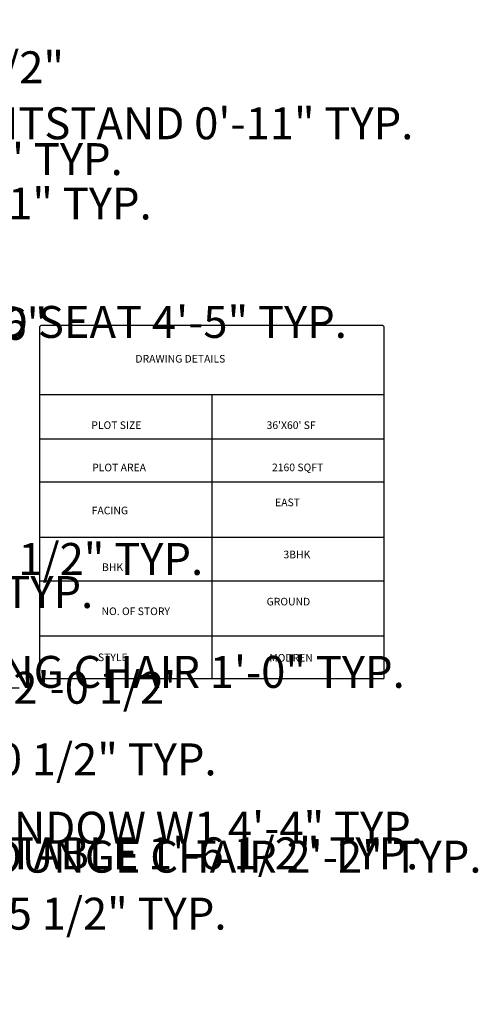
# Model space of a CAD drawing. Units: inches. Extents: x 35 to 5908, y 4 to 3165.
# Tile 6 of 6: x 5546 to 5908, y 2388 to 3165. Entities that reach past the tile are written whole.
import ezdxf

# ---------------------------------------------------------------- set-up
doc = ezdxf.new("R2010")
doc.units = ezdxf.units.IN
doc.header["$MEASUREMENT"] = 0
for name, color, linetype, lineweight in [('A-ANNO-DIMS', 2, 'Continuous', 18), ('A-ANNO-TEXT', 7, 'Continuous', 18), ('A-ANNO-TTLB', 7, 'Continuous', 25)]:
    doc.layers.add(name, color=color, linetype=linetype, lineweight=lineweight)
doc.styles.get("Standard").update_dxf_attribs({"font": 'arial.ttf'})
doc.dimstyles.get("Standard").update_dxf_attribs({"dimtxt": 25.18, "dimasz": 25.18, "dimexe": 0.18, "dimexo": 0.0625, "dimgap": 0.09, "dimtad": 0, "dimtih": 1, "dimtoh": 1, "dimdec": 0, "dimzin": 0, "dimdsep": 46, "dimlunit": 3, "dimtxsty": 'Standard', "dimcen": 0.09, "dimadec": 0, "dimazin": 0, "dimtfac": 1, "dimtdec": 0, "dimtofl": 0, "dimtmove": 0, "dimatfit": 3, "dimfxl": 1, "dimtolj": 1, "dimtzin": 0, "dimarcsym": 0})

# ---------------------------------------------------------------- blocks, each defined once
blk = doc.blocks.new('*D20')
at = {"layer": 'A-ANNO-DIMS', "color": 0, "lineweight": -2, "transparency": 16777216}
for p, q in [((5366.93, 2650.28), (5341.75, 2650.28)), ((5392.11, 2652.05), (5392.11, 2650.1)), ((5404.3, 2652.05), (5404.3, 2650.1)), ((5429.48, 2650.28), (5454.66, 2650.28))]:
    blk.add_line(p, q, dxfattribs=at)
for points in [[(5366.93, 2654.48), (5366.93, 2646.08), (5392.11, 2650.28)], [(5429.48, 2654.48), (5429.48, 2646.08), (5404.3, 2650.28)]]:
    blk.add_solid(points, dxfattribs=at)
at = {"layer": 'Defpoints', "color": 0, "lineweight": -2, "transparency": 16777216}
for p in [(5392.11, 2652.11), (5404.3, 2652.11), (5404.3, 2650.28)]:
    blk.add_point(p, dxfattribs=at)
at = {"layer": 'A-ANNO-DIMS', "color": 0, "transparency": 16777216, "insert": (5656.92, 2650.28), "char_height": 25.18, "attachment_point": 5}
blk.add_mtext('\\A1;DINING CHAIR 1\'-0" TYP.', dxfattribs=at)
blk = doc.blocks.new('*D21')
at = {"layer": 'A-ANNO-DIMS', "color": 0, "lineweight": -2, "transparency": 16777216}
for p, q in [((5406.13, 2688.06), (5406.13, 2713.24)), ((5406.13, 2713.24), (5431.31, 2713.24)), ((5404.36, 2662.88), (5406.31, 2662.88)), ((5404.36, 2652.11), (5406.31, 2652.11)), ((5406.13, 2626.93), (5406.13, 2601.75))]:
    blk.add_line(p, q, dxfattribs=at)
for points in [[(5401.93, 2688.06), (5410.32, 2688.06), (5406.13, 2662.88)], [(5401.93, 2626.93), (5410.32, 2626.93), (5406.13, 2652.11)]]:
    blk.add_solid(points, dxfattribs=at)
at = {"layer": 'Defpoints', "color": 0, "lineweight": -2, "transparency": 16777216}
for p in [(5404.3, 2662.88), (5406.13, 2662.88), (5404.3, 2652.11)]:
    blk.add_point(p, dxfattribs=at)
at = {"layer": 'A-ANNO-DIMS', "color": 0, "transparency": 16777216, "insert": (5517.92, 2713.24), "char_height": 25.18, "attachment_point": 5}
blk.add_mtext('\\A1;0\'-11" TYP.', dxfattribs=at)
blk = doc.blocks.new('*D22')
at = {"layer": 'A-ANNO-DIMS', "color": 0, "lineweight": -2, "transparency": 16777216}
for p, q in [((5466.99, 2502.2), (5466.99, 2527.38)), ((5466.99, 2527.38), (5492.17, 2527.38)), ((5474.73, 2502.2), (5466.81, 2502.2)), ((5466.99, 2475.38), (5466.99, 2477.02)), ((5474.73, 2450.2), (5466.81, 2450.2))]:
    blk.add_line(p, q, dxfattribs=at)
for points in [[(5462.8, 2477.02), (5471.19, 2477.02), (5466.99, 2502.2)], [(5462.8, 2475.38), (5471.19, 2475.38), (5466.99, 2450.2)]]:
    blk.add_solid(points, dxfattribs=at)
at = {"layer": 'Defpoints', "color": 0, "lineweight": -2, "transparency": 16777216}
for p in [(5466.99, 2502.2), (5474.79, 2502.2), (5474.79, 2450.2)]:
    blk.add_point(p, dxfattribs=at)
at = {"layer": 'A-ANNO-DIMS', "color": 0, "transparency": 16777216, "insert": (5682.85, 2527.38), "char_height": 25.18, "attachment_point": 5}
blk.add_mtext('\\A1;WINDOW W1 4\'-4" TYP.', dxfattribs=at)
blk = doc.blocks.new('*D32')
at = {"layer": 'A-ANNO-DIMS', "color": 0, "lineweight": -2, "transparency": 16777216}
for p, q in [((5230.02, 2744.72), (5230.02, 2739.16)), ((5266.29, 2744.72), (5266.29, 2739.16)), ((5204.84, 2739.34), (5179.66, 2739.34)), ((5291.47, 2739.34), (5316.65, 2739.34))]:
    blk.add_line(p, q, dxfattribs=at)
for points in [[(5204.84, 2743.53), (5204.84, 2735.14), (5230.02, 2739.34)], [(5291.47, 2743.53), (5291.47, 2735.14), (5266.29, 2739.34)]]:
    blk.add_solid(points, dxfattribs=at)
at = {"layer": 'Defpoints', "color": 0, "lineweight": -2, "transparency": 16777216}
for p in [(5230.02, 2744.78), (5266.29, 2744.78), (5266.29, 2739.34)]:
    blk.add_point(p, dxfattribs=at)
at = {"layer": 'A-ANNO-DIMS', "color": 0, "transparency": 16777216, "insert": (5507.22, 2739.34), "char_height": 25.18, "attachment_point": 5}
blk.add_mtext('\\A1;DOOR D3 3\'-0 1/2" TYP.', dxfattribs=at)
blk = doc.blocks.new('*D34')
at = {"layer": 'A-ANNO-DIMS', "color": 0, "lineweight": -2, "transparency": 16777216}
for p, q in [((5201.71, 3029.52), (5201.71, 3054.7)), ((5201.71, 3054.7), (5226.89, 3054.7)), ((5193.01, 3029.52), (5201.89, 3029.52)), ((5201.71, 2996.29), (5201.71, 3004.34)), ((5193.01, 2971.11), (5201.89, 2971.11))]:
    blk.add_line(p, q, dxfattribs=at)
for points in [[(5197.51, 3004.34), (5205.9, 3004.34), (5201.71, 3029.52)], [(5197.51, 2996.29), (5205.9, 2996.29), (5201.71, 2971.11)]]:
    blk.add_solid(points, dxfattribs=at)
at = {"layer": 'Defpoints', "color": 0, "lineweight": -2, "transparency": 16777216}
for p in [(5192.94, 3029.52), (5201.71, 3029.52), (5192.94, 2971.11)]:
    blk.add_point(p, dxfattribs=at)
at = {"layer": 'A-ANNO-DIMS', "color": 0, "transparency": 16777216, "insert": (5429.25, 3054.7), "char_height": 25.18, "attachment_point": 5}
blk.add_mtext('\\A1;BATHTUB 4\'-10 1/2" TYP.', dxfattribs=at)
blk = doc.blocks.new('*D36')
at = {"layer": 'A-ANNO-DIMS', "color": 0, "lineweight": -2, "transparency": 16777216}
for p, q in [((5428.75, 3057.76), (5428.75, 3082.94)), ((5428.75, 3082.94), (5453.93, 3082.94)), ((5427.13, 3032.58), (5428.93, 3032.58)), ((5427.13, 3021.38), (5428.93, 3021.38)), ((5428.75, 2996.2), (5428.75, 2971.02))]:
    blk.add_line(p, q, dxfattribs=at)
for points in [[(5424.55, 3057.76), (5432.94, 3057.76), (5428.75, 3032.58)], [(5424.55, 2996.2), (5432.94, 2996.2), (5428.75, 3021.38)]]:
    blk.add_solid(points, dxfattribs=at)
at = {"layer": 'Defpoints', "color": 0, "lineweight": -2, "transparency": 16777216}
for p in [(5427.07, 3032.58), (5428.75, 3032.58), (5427.07, 3021.38)]:
    blk.add_point(p, dxfattribs=at)
at = {"layer": 'A-ANNO-DIMS', "color": 0, "transparency": 16777216, "insert": (5659.14, 3082.94), "char_height": 25.18, "attachment_point": 5}
blk.add_mtext('\\A1;NIGHTSTAND 0\'-11" TYP.', dxfattribs=at)
blk = doc.blocks.new('*D37')
at = {"layer": 'A-ANNO-DIMS', "color": 0, "lineweight": -2, "transparency": 16777216}
for p, q in [((5415.94, 3021.32), (5415.94, 3019.52)), ((5427.07, 3021.32), (5427.07, 3019.52)), ((5390.76, 3019.7), (5365.58, 3019.7)), ((5452.25, 3019.7), (5477.43, 3019.7))]:
    blk.add_line(p, q, dxfattribs=at)
for points in [[(5390.76, 3023.9), (5390.76, 3015.51), (5415.94, 3019.7)], [(5452.25, 3023.9), (5452.25, 3015.51), (5427.07, 3019.7)]]:
    blk.add_solid(points, dxfattribs=at)
at = {"layer": 'Defpoints', "color": 0, "lineweight": -2, "transparency": 16777216}
for p in [(5415.94, 3021.38), (5427.07, 3021.38), (5427.07, 3019.7)]:
    blk.add_point(p, dxfattribs=at)
at = {"layer": 'A-ANNO-DIMS', "color": 0, "transparency": 16777216, "insert": (5564.04, 3019.7), "char_height": 25.18, "attachment_point": 5}
blk.add_mtext('\\A1;0\'-11" TYP.', dxfattribs=at)
blk = doc.blocks.new('*D40')
at = {"layer": 'A-ANNO-DIMS', "color": 0, "lineweight": -2, "transparency": 16777216}
for p, q in [((5327.75, 2918.38), (5327.75, 2926.45)), ((5352.93, 2926.27), (5355.55, 2926.27)), ((5380.73, 2918.38), (5380.73, 2926.45)), ((5380.73, 2926.27), (5405.91, 2926.27))]:
    blk.add_line(p, q, dxfattribs=at)
for points in [[(5352.93, 2930.46), (5352.93, 2922.07), (5327.75, 2926.27)], [(5355.55, 2930.46), (5355.55, 2922.07), (5380.73, 2926.27)]]:
    blk.add_solid(points, dxfattribs=at)
at = {"layer": 'Defpoints', "color": 0, "lineweight": -2, "transparency": 16777216}
for p in [(5380.73, 2926.27), (5327.75, 2918.32), (5380.73, 2918.32)]:
    blk.add_point(p, dxfattribs=at)
at = {"layer": 'A-ANNO-DIMS', "color": 0, "transparency": 16777216, "insert": (5612.58, 2926.27), "char_height": 25.18, "attachment_point": 5}
blk.add_mtext('\\A1;CURVED SEAT 4\'-5" TYP.', dxfattribs=at)
blk = doc.blocks.new('*D42')
at = {"layer": 'A-ANNO-DIMS', "color": 0, "lineweight": -2, "transparency": 16777216}
for p, q in [((5390.78, 2504.54), (5365.6, 2504.54)), ((5415.96, 2508.34), (5415.96, 2504.36)), ((5441.72, 2508.34), (5441.72, 2504.36)), ((5466.9, 2504.54), (5492.08, 2504.54))]:
    blk.add_line(p, q, dxfattribs=at)
for points in [[(5390.78, 2508.73), (5390.78, 2500.34), (5415.96, 2504.54)], [(5466.9, 2508.73), (5466.9, 2500.34), (5441.72, 2504.54)]]:
    blk.add_solid(points, dxfattribs=at)
at = {"layer": 'Defpoints', "color": 0, "lineweight": -2, "transparency": 16777216}
for p in [(5415.96, 2508.4), (5441.72, 2508.4), (5441.72, 2504.54)]:
    blk.add_point(p, dxfattribs=at)
at = {"layer": 'A-ANNO-DIMS', "color": 0, "transparency": 16777216, "insert": (5707.13, 2504.54), "char_height": 25.18, "attachment_point": 5}
blk.add_mtext('\\A1;LOUNGE CHAIR 2\'-2" TYP.', dxfattribs=at)
blk = doc.blocks.new('*D43')
at = {"layer": 'A-ANNO-DIMS', "color": 0, "lineweight": -2, "transparency": 16777216}
for p, q in [((5445.59, 2556.09), (5445.59, 2581.27)), ((5445.59, 2581.27), (5470.77, 2581.27)), ((5441.78, 2530.91), (5445.77, 2530.91)), ((5441.78, 2508.4), (5445.77, 2508.4)), ((5445.59, 2483.22), (5445.59, 2458.04))]:
    blk.add_line(p, q, dxfattribs=at)
for points in [[(5441.39, 2556.09), (5449.78, 2556.09), (5445.59, 2530.91)], [(5441.39, 2483.22), (5449.78, 2483.22), (5445.59, 2508.4)]]:
    blk.add_solid(points, dxfattribs=at)
at = {"layer": 'Defpoints', "color": 0, "lineweight": -2, "transparency": 16777216}
for p in [(5441.72, 2530.91), (5445.59, 2530.91), (5441.72, 2508.4)]:
    blk.add_point(p, dxfattribs=at)
at = {"layer": 'A-ANNO-DIMS', "color": 0, "transparency": 16777216, "insert": (5585.53, 2581.27), "char_height": 25.18, "attachment_point": 5}
blk.add_mtext('\\A1;1\'-10 1/2" TYP.', dxfattribs=at)
blk = doc.blocks.new('*D44')
at = {"layer": 'A-ANNO-DIMS', "color": 0, "lineweight": -2, "transparency": 16777216}
for p, q in [((5427.23, 2481.99), (5427.23, 2507.17)), ((5427.23, 2507.17), (5452.41, 2507.17)), ((5429.92, 2456.81), (5427.05, 2456.81)), ((5429.92, 2438.45), (5427.05, 2438.45)), ((5427.23, 2413.27), (5427.23, 2388.09))]:
    blk.add_line(p, q, dxfattribs=at)
for points in [[(5423.03, 2481.99), (5431.43, 2481.99), (5427.23, 2456.81)], [(5423.03, 2413.27), (5431.43, 2413.27), (5427.23, 2438.45)]]:
    blk.add_solid(points, dxfattribs=at)
at = {"layer": 'Defpoints', "color": 0, "lineweight": -2, "transparency": 16777216}
for p in [(5427.23, 2456.81), (5429.99, 2456.81), (5429.99, 2438.45)]:
    blk.add_point(p, dxfattribs=at)
at = {"layer": 'A-ANNO-DIMS', "color": 0, "transparency": 16777216, "insert": (5660.55, 2507.17), "char_height": 25.18, "attachment_point": 5}
blk.add_mtext('\\A1;END TABLE 1\'-6 1/2" TYP.', dxfattribs=at)
blk = doc.blocks.new('*D45')
at = {"layer": 'A-ANNO-DIMS', "color": 0, "lineweight": -2, "transparency": 16777216}
for p, q in [((5404.81, 2459.57), (5379.63, 2459.57)), ((5429.99, 2456.88), (5429.99, 2459.75)), ((5447.54, 2456.88), (5447.54, 2459.75)), ((5472.72, 2459.57), (5497.9, 2459.57))]:
    blk.add_line(p, q, dxfattribs=at)
for points in [[(5404.81, 2463.77), (5404.81, 2455.37), (5429.99, 2459.57)], [(5472.72, 2463.77), (5472.72, 2455.37), (5447.54, 2459.57)]]:
    blk.add_solid(points, dxfattribs=at)
at = {"layer": 'Defpoints', "color": 0, "lineweight": -2, "transparency": 16777216}
for p in [(5429.99, 2456.81), (5447.54, 2459.57), (5447.54, 2456.81)]:
    blk.add_point(p, dxfattribs=at)
at = {"layer": 'A-ANNO-DIMS', "color": 0, "transparency": 16777216, "insert": (5602.88, 2459.57), "char_height": 25.18, "attachment_point": 5}
blk.add_mtext('\\A1;1\'-5 1/2" TYP.', dxfattribs=at)
blk = doc.blocks.new('*D47')
at = {"layer": 'A-ANNO-DIMS', "color": 0, "lineweight": -2, "transparency": 16777216}
for p, q in [((5480.86, 3041.78), (5520.82, 3041.78)), ((5520.64, 3016.6), (5520.64, 2937.73)), ((5520.64, 2832.96), (5520.64, 2911.83)), ((5474.86, 2807.78), (5520.82, 2807.78))]:
    blk.add_line(p, q, dxfattribs=at)
for points in [[(5516.45, 3016.6), (5524.84, 3016.6), (5520.64, 3041.78)], [(5516.45, 2832.96), (5524.84, 2832.96), (5520.64, 2807.78)]]:
    blk.add_solid(points, dxfattribs=at)
at = {"layer": 'Defpoints', "color": 0, "lineweight": -2, "transparency": 16777216}
for p in [(5480.79, 3041.78), (5474.79, 2807.78), (5520.64, 2807.78)]:
    blk.add_point(p, dxfattribs=at)
at = {"layer": 'A-ANNO-DIMS', "color": 0, "transparency": 16777216, "insert": (5520.64, 2924.78), "char_height": 25.18, "attachment_point": 5}
blk.add_mtext('\\A1;19\'-6"', dxfattribs=at)
blk = doc.blocks.new('*D50')
at = {"layer": 'A-ANNO-DIMS', "color": 0, "lineweight": -2, "transparency": 16777216}
for p, q in [((5269.79, 2562.84), (5269.79, 3127.3)), ((5294.97, 3127.12), (5382.35, 3127.12)), ((5407.53, 2562.84), (5407.53, 3127.3)), ((5407.53, 3127.12), (5432.71, 3127.12))]:
    blk.add_line(p, q, dxfattribs=at)
for points in [[(5294.97, 3131.32), (5294.97, 3122.92), (5269.79, 3127.12)], [(5382.35, 3131.32), (5382.35, 3122.92), (5407.53, 3127.12)]]:
    blk.add_solid(points, dxfattribs=at)
at = {"layer": 'Defpoints', "color": 0, "lineweight": -2, "transparency": 16777216}
for p in [(5407.53, 3127.12), (5269.79, 2562.78), (5407.53, 2562.78)]:
    blk.add_point(p, dxfattribs=at)
at = {"layer": 'A-ANNO-DIMS', "color": 0, "transparency": 16777216, "insert": (5504.2, 3127.12), "char_height": 25.18, "attachment_point": 5}
blk.add_mtext('\\A1;11\'-5 1/2"', dxfattribs=at)
blk = doc.blocks.new('*D51')
at = {"layer": 'A-ANNO-DIMS', "color": 0, "lineweight": -2, "transparency": 16777216}
for p, q in [((5520.64, 2612.59), (5520.64, 2637.77)), ((5520.64, 2637.77), (5545.82, 2637.77)), ((5407.59, 2587.41), (5520.82, 2587.41)), ((5407.59, 2562.78), (5520.82, 2562.78)), ((5520.64, 2537.6), (5520.64, 2512.42))]:
    blk.add_line(p, q, dxfattribs=at)
for points in [[(5516.45, 2612.59), (5524.84, 2612.59), (5520.64, 2587.41)], [(5516.45, 2537.6), (5524.84, 2537.6), (5520.64, 2562.78)]]:
    blk.add_solid(points, dxfattribs=at)
at = {"layer": 'Defpoints', "color": 0, "lineweight": -2, "transparency": 16777216}
for p in [(5407.53, 2587.41), (5520.64, 2587.41), (5407.53, 2562.78)]:
    blk.add_point(p, dxfattribs=at)
at = {"layer": 'A-ANNO-DIMS', "color": 0, "transparency": 16777216, "insert": (5608.93, 2637.77), "char_height": 25.18, "attachment_point": 5}
blk.add_mtext('\\A1;2\'-0 1/2"', dxfattribs=at)

msp = doc.modelspace()

# ---------------------------------------------------------------- linework, layer by layer
at = {"layer": 'A-ANNO-TTLB'}
for p, q in [((5562.14, 2868.99), (5833.45, 2868.99)), ((5697.8, 2868.99), (5697.8, 2678.68)), ((5562.14, 2834.15), (5833.45, 2834.15)), ((5562.14, 2800.27), (5833.45, 2800.27)), ((5562.14, 2756.54), (5833.45, 2756.54)), ((5562.14, 2722.06), (5833.45, 2722.06)), ((5562.14, 2678.68), (5833.45, 2678.68)), ((5697.8, 2678.68), (5697.8, 2645.09)), ((5562.14, 2645.09), (5833.45, 2645.09))]:
    msp.add_line(p, q, dxfattribs=at)
msp.add_lwpolyline([(5562.14, 2645.09), (5562.14, 2921.79, -0.414214), (5564.14, 2923.79), (5831.45, 2923.79, -0.414214), (5833.45, 2921.79), (5833.45, 2645.09)], format="xyb", dxfattribs=at)

# ---------------------------------------------------------------- texts
at = {"layer": 'A-ANNO-TEXT', "char_height": 6, "attachment_point": 1}
for s, insert in [('DRAWING DETAILS', (5637.57, 2900.22)), ('PLOT SIZE', (5602.79, 2847.86)), ("36'X60' SF", (5740.98, 2847.86)), ('PLOT AREA', (5603.5, 2814.47)), ('2160 SQFT', (5745.22, 2814.56)), ('FACING', (5603.12, 2780.55)), ('EAST', (5747.68, 2786.97)), ('3BHK', (5754.26, 2745.86)), ('BHK', (5611.24, 2735.88)), ('GROUND', (5740.98, 2708.7)), ('NO. OF STORY', (5610.87, 2701.08)), ('STYLE', (5608.02, 2664.77)), ('MODREN', (5743.07, 2664.38))]:
    msp.add_mtext_dynamic_manual_height_columns(s, width=168.2079, gutter_width=1, heights=[0], dxfattribs=dict(at, insert=insert))

# ---------------------------------------------------------------- dimensions: what is measured, and where the dimension line sits
at = {"layer": 'A-ANNO-DIMS'}
dim = msp.add_linear_dim(base=(5407.53, 3127.12), p1=(5269.79, 2562.78), p2=(5407.53, 2562.78), dimstyle='Standard', override={"dimdec": 1, "dimlfac": 1, "dimrnd": 0, "dimzin": 1, "dimdsep": 46, "dimlunit": 4, "dimfrac": 2}, dxfattribs=at)
dim.commit()
dim.dimension.update_dxf_attribs({"geometry": '*D50', "text_midpoint": (5504.2, 3127.12)})
for base, p1, p2, angle, text, picture, middle in [((5428.75, 3032.58), (5427.07, 3021.38), (5427.07, 3032.58), 90, 'NIGHTSTAND <> TYP.', '*D36', (5659.14, 3082.94)), ((5201.71, 3029.52), (5192.94, 2971.11), (5192.94, 3029.52), 90, 'BATHTUB <> TYP.', '*D34', (5429.25, 3054.7)), ((5380.73, 2926.27), (5327.75, 2918.32), (5380.73, 2918.32), 0, 'CURVED SEAT <> TYP.', '*D40', (5612.58, 2926.27)), ((5406.13, 2662.88), (5404.3, 2652.11), (5404.3, 2662.88), 90, '<> TYP.', '*D21', (5517.92, 2713.24)), ((5445.59, 2530.91), (5441.72, 2508.4), (5441.72, 2530.91), 90, '<> TYP.', '*D43', (5585.53, 2581.27)), ((5427.23, 2456.81), (5429.99, 2438.45), (5429.99, 2456.81), 90, 'END TABLE <> TYP.', '*D44', (5660.55, 2507.17)), ((5466.99, 2502.2), (5474.79, 2450.2), (5474.79, 2502.2), 90, 'WINDOW W1 <> TYP.', '*D22', (5682.85, 2527.38))]:
    dim = msp.add_linear_dim(base=base, p1=p1, p2=p2, angle=angle, text=text, dimstyle='Standard', override={"dimdec": 1, "dimlfac": 1, "dimrnd": 0, "dimzin": 1, "dimdsep": 46, "dimlunit": 4, "dimfrac": 2}, dxfattribs=at)
    dim.commit()
    dim.dimension.update_dxf_attribs({"geometry": picture, "text_midpoint": middle})
for base, p1, p2, text, picture, middle in [((5427.07, 3019.7), (5415.94, 3021.38), (5427.07, 3021.38), '<> TYP.', '*D37', (5564.04, 3019.7)), ((5266.29, 2739.34), (5230.02, 2744.78), (5266.29, 2744.78), 'DOOR D3 <> TYP.', '*D32', (5507.22, 2739.34)), ((5404.3, 2650.28), (5392.11, 2652.11), (5404.3, 2652.11), 'DINING CHAIR <> TYP.', '*D20', (5656.92, 2650.28)), ((5441.72, 2504.54), (5415.96, 2508.4), (5441.72, 2508.4), 'LOUNGE CHAIR <> TYP.', '*D42', (5707.13, 2504.54)), ((5447.5359, 2459.5686), (5429.9857, 2456.8141), (5447.5359, 2456.8141), '<> TYP.', '*D45', (5602.8797, 2459.5686))]:
    dim = msp.add_linear_dim(base=base, p1=p1, p2=p2, text=text, dimstyle='Standard', override={"dimdec": 1, "dimlfac": 1, "dimrnd": 0, "dimzin": 1, "dimdsep": 46, "dimlunit": 4, "dimfrac": 2}, dxfattribs=at)
    dim.commit()
    dim.dimension.update_dxf_attribs({"geometry": picture, "text_midpoint": middle})
for base, p1, p2, picture, middle in [((5520.64, 2807.78), (5480.79, 3041.78), (5474.79, 2807.78), '*D47', (5520.64, 2924.78)), ((5520.64, 2587.41), (5407.53, 2562.78), (5407.53, 2587.41), '*D51', (5608.93, 2637.77))]:
    dim = msp.add_linear_dim(base=base, p1=p1, p2=p2, angle=90, dimstyle='Standard', override={"dimdec": 1, "dimlfac": 1, "dimrnd": 0, "dimzin": 1, "dimdsep": 46, "dimlunit": 4, "dimfrac": 2}, dxfattribs=at)
    dim.commit()
    dim.dimension.update_dxf_attribs({"geometry": picture, "text_midpoint": middle})

doc.saveas('drawing.dxf')
